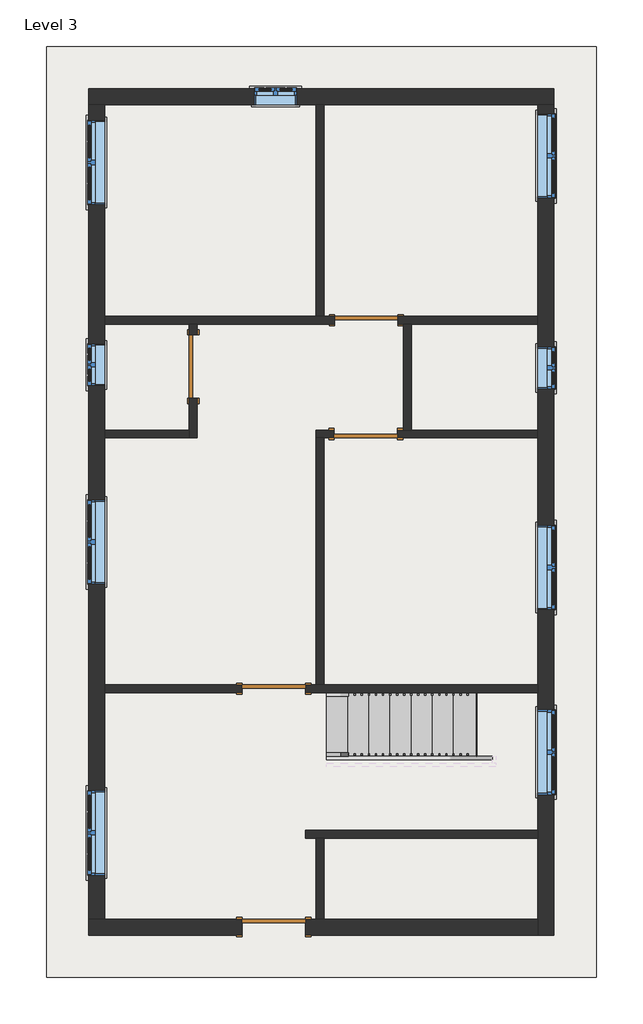
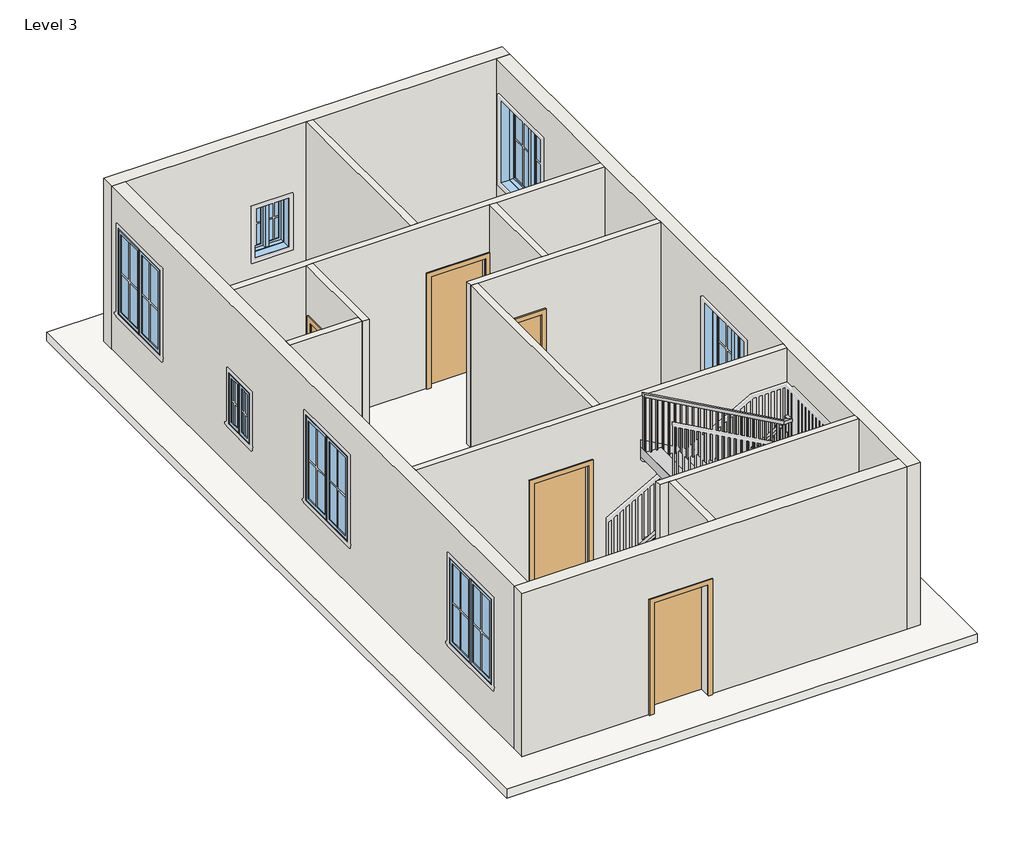
# One storey, part 1 of 2: 14 walls, 9 windows, 5 doors, 1 railing, 1 roof, 1 stair flight.
"""IFC4 building model written with IfcOpenShell, lengths in millimetres."""

from ifc_helpers import new_model, si_unit, frame, origin, place, context, project, spatial, polyline, outline, extrude, faceted_brep, transform, mapped, element, save
from components import door_305aa2a5, door_e5f9f3c4, door_a90ba1ad, stair_flight_ef7e9c63, window_c417fced, window_8377141f

model = new_model("IFC4")

# Units and contexts
model_context = context("Model", 3, world=origin())
ifc_project = project(units=[si_unit("LENGTHUNIT", "METRE", prefix="MILLI")], contexts=[model_context])

# Site, building, storey
site = spatial("IfcSite", under=ifc_project)
building = spatial("IfcBuilding", under=site)
storey = spatial("IfcBuildingStorey", under=building, Name="Level 3", Elevation=6096.0)

# Doors
placement = place(None, origin())
door_shape = door_305aa2a5(model_context)
element("IfcDoor", 1, ObjectType="Single-Flush : 36\" x 84\"", at=placement, inside=storey, context=model_context, shape_type="MappedRepresentation", body=[
    mapped(door_shape, transform((5270.5, 10636.25, 6096.0), x_axis=(-1.0, 0.0, 0.0), y_axis=(0.0, -1.0, 0.0), z_axis=(0.0, 0.0, 1.0))),
])
door_2_shape = door_e5f9f3c4(model_context)
element("IfcDoor", 2, ObjectType="Single-Flush : 36\" x 84\"", at=placement, inside=storey, context=model_context, shape_type="MappedRepresentation", body=[
    mapped(door_2_shape, transform((2774.95, 9969.5, 6096.0), x_axis=(0.0, 1.0, 0.0), y_axis=(-1.0, 0.0, 0.0), z_axis=(0.0, 0.0, 1.0))),
])
element("IfcDoor", 3, ObjectType="Single-Flush : 36\" x 84\"", at=placement, inside=storey, context=model_context, shape_type="MappedRepresentation", body=[
    mapped(door_2_shape, transform((5264.15, 8997.95, 6096.0), x_axis=(-1.0, 0.0, 0.0), y_axis=(0.0, -1.0, 0.0), z_axis=(0.0, 0.0, 1.0))),
])
element("IfcDoor", 4, ObjectType="Single-Flush : 36\" x 84\"", at=placement, inside=storey, context=model_context, shape_type="MappedRepresentation", body=[
    mapped(door_2_shape, transform((3937.0, 5327.65, 6096.0), x_axis=(1.0, 0.0, 0.0), y_axis=(0.0, 1.0, 0.0), z_axis=(0.0, 0.0, 1.0))),
])
door_3_shape = door_a90ba1ad(model_context)
element("IfcDoor", 5, ObjectType="Single-Flush : 36\" x 84\"", at=placement, inside=storey, context=model_context, shape_type="MappedRepresentation", body=[
    mapped(door_3_shape, transform((3937.0, 1892.3, 6096.0), x_axis=(-1.0, 0.0, 0.0), y_axis=(0.0, -1.0, 0.0), z_axis=(0.0, 0.0, 1.0))),
])

# Railing
element("IfcRailing", 6, ObjectType="Handrail - Rectangular", at=placement, inside=storey, context=model_context, shape_type="SolidModel", body=[
    faceted_brep([(4699.0, 4406.9, 7179.7333333), (4699.0, 4406.9, 7121.620221), (4699.0, 4356.1, 7121.620221), (4699.0, 4356.1, 7179.7333333), (7061.2, 4406.9, 8492.0666667), (7112.0, 4406.9, 8462.1757765), (7112.0, 4356.1, 8462.1757765), (7061.2, 4356.1, 8492.0666667), (7061.2, 4406.9, 8534.4), (7112.0, 4406.9, 8483.6), (7112.0, 4356.1, 8483.6), (7061.2, 4356.1, 8534.4), (7188.2, 4406.9, 8534.4), (7188.2, 4406.9, 8483.6), (7137.4, 4356.1, 8483.6), (7137.4, 4356.1, 8534.4), (7188.2, 4279.9, 8534.4), (7188.2, 4229.1, 8483.6), (7137.4, 4229.1, 8483.6), (7137.4, 4279.9, 8534.4), (7188.2, 4279.9, 8746.0666667), (7188.2, 4229.1, 8695.2666667), (7137.4, 4229.1, 8695.2666667), (7137.4, 4279.9, 8746.0666667), (7188.2, 4152.9, 8746.0666667), (7188.2, 4152.9, 8695.2666667), (7137.4, 4203.7, 8695.2666667), (7137.4, 4203.7, 8746.0666667), (7061.2, 4152.9, 8746.0666667), (7048.0363978, 4152.9, 8695.2666667), (7048.0363978, 4203.7, 8695.2666667), (7061.2, 4203.7, 8746.0666667), (4699.0, 4152.9, 10058.4), (4699.0, 4203.7, 10058.4), (4699.0, 4203.7, 10000.2868876), (4699.0, 4152.9, 10000.2868876)], [[[0, 1, 2, 3]], [[1, 0, 4, 5]], [[2, 1, 5, 6]], [[3, 2, 6, 7]], [[0, 3, 7, 4]], [[5, 4, 8, 9]], [[6, 5, 9, 10]], [[7, 6, 10, 11]], [[4, 7, 11, 8]], [[9, 8, 12, 13]], [[10, 9, 13, 14]], [[11, 10, 14, 15]], [[8, 11, 15, 12]], [[13, 12, 16, 17]], [[14, 13, 17, 18]], [[15, 14, 18, 19]], [[12, 15, 19, 16]], [[17, 16, 20, 21]], [[18, 17, 21, 22]], [[19, 18, 22, 23]], [[16, 19, 23, 20]], [[21, 20, 24, 25]], [[22, 21, 25, 26]], [[23, 22, 26, 27]], [[20, 23, 27, 24]], [[25, 24, 28, 29]], [[26, 25, 29, 30]], [[27, 26, 30, 31]], [[24, 27, 31, 28]], [[32, 33, 34, 35]], [[29, 28, 32, 35]], [[30, 29, 35, 34]], [[31, 30, 34, 33]], [[28, 31, 33, 32]]]),
    extrude(outline(polyline([(9980.8841099, 4733.925), (9991.4674432, 4714.875), (8974.6666667, 4714.875), (8974.6666667, 4733.925), (9980.8841099, 4733.925)])), frame((0.0, 4168.775, 0.0), z_axis=(0.0, 1.0, 0.0), x_axis=(0.0, 0.0, 1.0)), (0.0, 0.0, 1.0), 19.05),
    extrude(outline(polyline([(9924.4396654, 4835.525), (9935.0229988, 4816.475), (8974.6666667, 4816.475), (8974.6666667, 4835.525), (9924.4396654, 4835.525)])), frame((0.0, 4168.775, 0.0), z_axis=(0.0, 1.0, 0.0), x_axis=(0.0, 0.0, 1.0)), (0.0, 0.0, 1.0), 19.05),
    extrude(outline(polyline([(9867.995221, 4937.125), (9878.5785543, 4918.075), (8974.6666667, 4918.075), (8974.6666667, 4937.125), (9867.995221, 4937.125)])), frame((0.0, 4168.775, 0.0), z_axis=(0.0, 1.0, 0.0), x_axis=(0.0, 0.0, 1.0)), (0.0, 0.0, 1.0), 19.05),
    extrude(outline(polyline([(9811.5507765, 5038.725), (9822.1341099, 5019.675), (8805.3333333, 5019.675), (8805.3333333, 5038.725), (9811.5507765, 5038.725)])), frame((0.0, 4168.775, 0.0), z_axis=(0.0, 1.0, 0.0), x_axis=(0.0, 0.0, 1.0)), (0.0, 0.0, 1.0), 19.05),
    extrude(outline(polyline([(9755.1063321, 5140.325), (9765.6896654, 5121.275), (8805.3333333, 5121.275), (8805.3333333, 5140.325), (9755.1063321, 5140.325)])), frame((0.0, 4168.775, 0.0), z_axis=(0.0, 1.0, 0.0), x_axis=(0.0, 0.0, 1.0)), (0.0, 0.0, 1.0), 19.05),
    extrude(outline(polyline([(9698.6618876, 5241.925), (9709.245221, 5222.875), (8805.3333333, 5222.875), (8805.3333333, 5241.925), (9698.6618876, 5241.925)])), frame((0.0, 4168.775, 0.0), z_axis=(0.0, 1.0, 0.0), x_axis=(0.0, 0.0, 1.0)), (0.0, 0.0, 1.0), 19.05),
    extrude(outline(polyline([(9642.2174432, 5343.525), (9652.8007765, 5324.475), (8636.0, 5324.475), (8636.0, 5343.525), (9642.2174432, 5343.525)])), frame((0.0, 4168.775, 0.0), z_axis=(0.0, 1.0, 0.0), x_axis=(0.0, 0.0, 1.0)), (0.0, 0.0, 1.0), 19.05),
    extrude(outline(polyline([(9585.7729988, 5445.125), (9596.3563321, 5426.075), (8636.0, 5426.075), (8636.0, 5445.125), (9585.7729988, 5445.125)])), frame((0.0, 4168.775, 0.0), z_axis=(0.0, 1.0, 0.0), x_axis=(0.0, 0.0, 1.0)), (0.0, 0.0, 1.0), 19.05),
    extrude(outline(polyline([(9529.3285543, 5546.725), (9539.9118876, 5527.675), (8636.0, 5527.675), (8636.0, 5546.725), (9529.3285543, 5546.725)])), frame((0.0, 4168.775, 0.0), z_axis=(0.0, 1.0, 0.0), x_axis=(0.0, 0.0, 1.0)), (0.0, 0.0, 1.0), 19.05),
    extrude(outline(polyline([(9472.8841099, 5648.325), (9483.4674432, 5629.275), (8466.6666667, 5629.275), (8466.6666667, 5648.325), (9472.8841099, 5648.325)])), frame((0.0, 4168.775, 0.0), z_axis=(0.0, 1.0, 0.0), x_axis=(0.0, 0.0, 1.0)), (0.0, 0.0, 1.0), 19.05),
    extrude(outline(polyline([(9416.4396654, 5749.925), (9427.0229988, 5730.875), (8466.6666667, 5730.875), (8466.6666667, 5749.925), (9416.4396654, 5749.925)])), frame((0.0, 4168.775, 0.0), z_axis=(0.0, 1.0, 0.0), x_axis=(0.0, 0.0, 1.0)), (0.0, 0.0, 1.0), 19.05),
    extrude(outline(polyline([(9359.995221, 5851.525), (9370.5785543, 5832.475), (8466.6666667, 5832.475), (8466.6666667, 5851.525), (9359.995221, 5851.525)])), frame((0.0, 4168.775, 0.0), z_axis=(0.0, 1.0, 0.0), x_axis=(0.0, 0.0, 1.0)), (0.0, 0.0, 1.0), 19.05),
    extrude(outline(polyline([(9303.5507765, 5953.125), (9314.1341099, 5934.075), (8297.3333333, 5934.075), (8297.3333333, 5953.125), (9303.5507765, 5953.125)])), frame((0.0, 4168.775, 0.0), z_axis=(0.0, 1.0, 0.0), x_axis=(0.0, 0.0, 1.0)), (0.0, 0.0, 1.0), 19.05),
    extrude(outline(polyline([(9247.1063321, 6054.725), (9257.6896654, 6035.675), (8297.3333333, 6035.675), (8297.3333333, 6054.725), (9247.1063321, 6054.725)])), frame((0.0, 4168.775, 0.0), z_axis=(0.0, 1.0, 0.0), x_axis=(0.0, 0.0, 1.0)), (0.0, 0.0, 1.0), 19.05),
    extrude(outline(polyline([(9190.6618876, 6156.325), (9201.245221, 6137.275), (8297.3333333, 6137.275), (8297.3333333, 6156.325), (9190.6618876, 6156.325)])), frame((0.0, 4168.775, 0.0), z_axis=(0.0, 1.0, 0.0), x_axis=(0.0, 0.0, 1.0)), (0.0, 0.0, 1.0), 19.05),
    extrude(outline(polyline([(9134.2174432, 6257.925), (9144.8007765, 6238.875), (8128.0, 6238.875), (8128.0, 6257.925), (9134.2174432, 6257.925)])), frame((0.0, 4168.775, 0.0), z_axis=(0.0, 1.0, 0.0), x_axis=(0.0, 0.0, 1.0)), (0.0, 0.0, 1.0), 19.05),
    extrude(outline(polyline([(9077.7729988, 6359.525), (9088.3563321, 6340.475), (8128.0, 6340.475), (8128.0, 6359.525), (9077.7729988, 6359.525)])), frame((0.0, 4168.775, 0.0), z_axis=(0.0, 1.0, 0.0), x_axis=(0.0, 0.0, 1.0)), (0.0, 0.0, 1.0), 19.05),
    extrude(outline(polyline([(9021.3285543, 6461.125), (9031.9118876, 6442.075), (8128.0, 6442.075), (8128.0, 6461.125), (9021.3285543, 6461.125)])), frame((0.0, 4168.775, 0.0), z_axis=(0.0, 1.0, 0.0), x_axis=(0.0, 0.0, 1.0)), (0.0, 0.0, 1.0), 19.05),
    extrude(outline(polyline([(8964.8841099, 6562.725), (8975.4674432, 6543.675), (7958.6666667, 6543.675), (7958.6666667, 6562.725), (8964.8841099, 6562.725)])), frame((0.0, 4168.775, 0.0), z_axis=(0.0, 1.0, 0.0), x_axis=(0.0, 0.0, 1.0)), (0.0, 0.0, 1.0), 19.05),
    extrude(outline(polyline([(8908.4396654, 6664.325), (8919.0229988, 6645.275), (7958.6666667, 6645.275), (7958.6666667, 6664.325), (8908.4396654, 6664.325)])), frame((0.0, 4168.775, 0.0), z_axis=(0.0, 1.0, 0.0), x_axis=(0.0, 0.0, 1.0)), (0.0, 0.0, 1.0), 19.05),
    extrude(outline(polyline([(8851.995221, 6765.925), (8862.5785543, 6746.875), (7958.6666667, 6746.875), (7958.6666667, 6765.925), (8851.995221, 6765.925)])), frame((0.0, 4168.775, 0.0), z_axis=(0.0, 1.0, 0.0), x_axis=(0.0, 0.0, 1.0)), (0.0, 0.0, 1.0), 19.05),
    extrude(outline(polyline([(8795.5507765, 6867.525), (8806.1341099, 6848.475), (7789.3333333, 6848.475), (7789.3333333, 6867.525), (8795.5507765, 6867.525)])), frame((0.0, 4168.775, 0.0), z_axis=(0.0, 1.0, 0.0), x_axis=(0.0, 0.0, 1.0)), (0.0, 0.0, 1.0), 19.05),
    extrude(outline(polyline([(8739.1063321, 6969.125), (8749.6896654, 6950.075), (7789.3333333, 6950.075), (7789.3333333, 6969.125), (8739.1063321, 6969.125)])), frame((0.0, 4168.775, 0.0), z_axis=(0.0, 1.0, 0.0), x_axis=(0.0, 0.0, 1.0)), (0.0, 0.0, 1.0), 19.05),
    extrude(outline(polyline([(8682.6618876, 7070.725), (8693.245221, 7051.675), (7789.3333333, 7051.675), (7789.3333333, 7070.725), (8682.6618876, 7070.725)])), frame((0.0, 4168.775, 0.0), z_axis=(0.0, 1.0, 0.0), x_axis=(0.0, 0.0, 1.0)), (0.0, 0.0, 1.0), 19.05),
    extrude(outline(polyline([(7153.275, 4289.425), (7172.325, 4289.425), (7172.325, 4270.375), (7153.275, 4270.375), (7153.275, 4289.425)])), frame((0.0, 0.0, 7620.0), z_axis=(0.0, 0.0, 1.0), x_axis=(1.0, 0.0, 0.0)), (0.0, 0.0, 1.0), 863.6),
    extrude(outline(polyline([(7127.875, 4371.975), (7127.875, 4391.025), (7146.925, 4391.025), (7146.925, 4371.975), (7127.875, 4371.975)])), frame((0.0, 0.0, 7620.0), z_axis=(0.0, 0.0, 1.0), x_axis=(1.0, 0.0, 0.0)), (0.0, 0.0, 1.0), 863.6),
    extrude(outline(polyline([(8425.1341099, 7045.325), (8414.5507765, 7026.275), (7450.6666667, 7026.275), (7450.6666667, 7045.325), (8425.1341099, 7045.325)])), frame((0.0, 4371.975, 0.0), z_axis=(0.0, 1.0, 0.0), x_axis=(0.0, 0.0, 1.0)), (0.0, 0.0, 1.0), 19.05),
    extrude(outline(polyline([(8368.6896654, 6943.725), (8358.1063321, 6924.675), (7450.6666667, 6924.675), (7450.6666667, 6943.725), (8368.6896654, 6943.725)])), frame((0.0, 4371.975, 0.0), z_axis=(0.0, 1.0, 0.0), x_axis=(0.0, 0.0, 1.0)), (0.0, 0.0, 1.0), 19.05),
    extrude(outline(polyline([(8312.245221, 6842.125), (8301.6618876, 6823.075), (7450.6666667, 6823.075), (7450.6666667, 6842.125), (8312.245221, 6842.125)])), frame((0.0, 4371.975, 0.0), z_axis=(0.0, 1.0, 0.0), x_axis=(0.0, 0.0, 1.0)), (0.0, 0.0, 1.0), 19.05),
    extrude(outline(polyline([(8255.8007765, 6740.525), (8245.2174432, 6721.475), (7281.3333333, 6721.475), (7281.3333333, 6740.525), (8255.8007765, 6740.525)])), frame((0.0, 4371.975, 0.0), z_axis=(0.0, 1.0, 0.0), x_axis=(0.0, 0.0, 1.0)), (0.0, 0.0, 1.0), 19.05),
    extrude(outline(polyline([(8199.3563321, 6638.925), (8188.7729988, 6619.875), (7281.3333333, 6619.875), (7281.3333333, 6638.925), (8199.3563321, 6638.925)])), frame((0.0, 4371.975, 0.0), z_axis=(0.0, 1.0, 0.0), x_axis=(0.0, 0.0, 1.0)), (0.0, 0.0, 1.0), 19.05),
    extrude(outline(polyline([(8142.9118876, 6537.325), (8132.3285543, 6518.275), (7281.3333333, 6518.275), (7281.3333333, 6537.325), (8142.9118876, 6537.325)])), frame((0.0, 4371.975, 0.0), z_axis=(0.0, 1.0, 0.0), x_axis=(0.0, 0.0, 1.0)), (0.0, 0.0, 1.0), 19.05),
    extrude(outline(polyline([(8086.4674432, 6435.725), (8075.8841099, 6416.675), (7112.0, 6416.675), (7112.0, 6435.725), (8086.4674432, 6435.725)])), frame((0.0, 4371.975, 0.0), z_axis=(0.0, 1.0, 0.0), x_axis=(0.0, 0.0, 1.0)), (0.0, 0.0, 1.0), 19.05),
    extrude(outline(polyline([(8030.0229988, 6334.125), (8019.4396654, 6315.075), (7112.0, 6315.075), (7112.0, 6334.125), (8030.0229988, 6334.125)])), frame((0.0, 4371.975, 0.0), z_axis=(0.0, 1.0, 0.0), x_axis=(0.0, 0.0, 1.0)), (0.0, 0.0, 1.0), 19.05),
    extrude(outline(polyline([(7973.5785543, 6232.525), (7962.995221, 6213.475), (7112.0, 6213.475), (7112.0, 6232.525), (7973.5785543, 6232.525)])), frame((0.0, 4371.975, 0.0), z_axis=(0.0, 1.0, 0.0), x_axis=(0.0, 0.0, 1.0)), (0.0, 0.0, 1.0), 19.05),
    extrude(outline(polyline([(7917.1341099, 6130.925), (7906.5507765, 6111.875), (6942.6666667, 6111.875), (6942.6666667, 6130.925), (7917.1341099, 6130.925)])), frame((0.0, 4371.975, 0.0), z_axis=(0.0, 1.0, 0.0), x_axis=(0.0, 0.0, 1.0)), (0.0, 0.0, 1.0), 19.05),
    extrude(outline(polyline([(7860.6896654, 6029.325), (7850.1063321, 6010.275), (6942.6666667, 6010.275), (6942.6666667, 6029.325), (7860.6896654, 6029.325)])), frame((0.0, 4371.975, 0.0), z_axis=(0.0, 1.0, 0.0), x_axis=(0.0, 0.0, 1.0)), (0.0, 0.0, 1.0), 19.05),
    extrude(outline(polyline([(7804.245221, 5927.725), (7793.6618876, 5908.675), (6942.6666667, 5908.675), (6942.6666667, 5927.725), (7804.245221, 5927.725)])), frame((0.0, 4371.975, 0.0), z_axis=(0.0, 1.0, 0.0), x_axis=(0.0, 0.0, 1.0)), (0.0, 0.0, 1.0), 19.05),
    extrude(outline(polyline([(7747.8007765, 5826.125), (7737.2174432, 5807.075), (6773.3333333, 5807.075), (6773.3333333, 5826.125), (7747.8007765, 5826.125)])), frame((0.0, 4371.975, 0.0), z_axis=(0.0, 1.0, 0.0), x_axis=(0.0, 0.0, 1.0)), (0.0, 0.0, 1.0), 19.05),
    extrude(outline(polyline([(7691.3563321, 5724.525), (7680.7729988, 5705.475), (6773.3333333, 5705.475), (6773.3333333, 5724.525), (7691.3563321, 5724.525)])), frame((0.0, 4371.975, 0.0), z_axis=(0.0, 1.0, 0.0), x_axis=(0.0, 0.0, 1.0)), (0.0, 0.0, 1.0), 19.05),
    extrude(outline(polyline([(7634.9118876, 5622.925), (7624.3285543, 5603.875), (6773.3333333, 5603.875), (6773.3333333, 5622.925), (7634.9118876, 5622.925)])), frame((0.0, 4371.975, 0.0), z_axis=(0.0, 1.0, 0.0), x_axis=(0.0, 0.0, 1.0)), (0.0, 0.0, 1.0), 19.05),
    extrude(outline(polyline([(7578.4674432, 5521.325), (7567.8841099, 5502.275), (6604.0, 5502.275), (6604.0, 5521.325), (7578.4674432, 5521.325)])), frame((0.0, 4371.975, 0.0), z_axis=(0.0, 1.0, 0.0), x_axis=(0.0, 0.0, 1.0)), (0.0, 0.0, 1.0), 19.05),
    extrude(outline(polyline([(7522.0229988, 5419.725), (7511.4396654, 5400.675), (6604.0, 5400.675), (6604.0, 5419.725), (7522.0229988, 5419.725)])), frame((0.0, 4371.975, 0.0), z_axis=(0.0, 1.0, 0.0), x_axis=(0.0, 0.0, 1.0)), (0.0, 0.0, 1.0), 19.05),
    extrude(outline(polyline([(7465.5785543, 5318.125), (7454.995221, 5299.075), (6604.0, 5299.075), (6604.0, 5318.125), (7465.5785543, 5318.125)])), frame((0.0, 4371.975, 0.0), z_axis=(0.0, 1.0, 0.0), x_axis=(0.0, 0.0, 1.0)), (0.0, 0.0, 1.0), 19.05),
    extrude(outline(polyline([(7409.1341099, 5216.525), (7398.5507765, 5197.475), (6434.6666667, 5197.475), (6434.6666667, 5216.525), (7409.1341099, 5216.525)])), frame((0.0, 4371.975, 0.0), z_axis=(0.0, 1.0, 0.0), x_axis=(0.0, 0.0, 1.0)), (0.0, 0.0, 1.0), 19.05),
    extrude(outline(polyline([(7352.6896654, 5114.925), (7342.1063321, 5095.875), (6434.6666667, 5095.875), (6434.6666667, 5114.925), (7352.6896654, 5114.925)])), frame((0.0, 4371.975, 0.0), z_axis=(0.0, 1.0, 0.0), x_axis=(0.0, 0.0, 1.0)), (0.0, 0.0, 1.0), 19.05),
    extrude(outline(polyline([(7296.245221, 5013.325), (7285.6618876, 4994.275), (6434.6666667, 4994.275), (6434.6666667, 5013.325), (7296.245221, 5013.325)])), frame((0.0, 4371.975, 0.0), z_axis=(0.0, 1.0, 0.0), x_axis=(0.0, 0.0, 1.0)), (0.0, 0.0, 1.0), 19.05),
    extrude(outline(polyline([(7239.8007765, 4911.725), (7229.2174432, 4892.675), (6265.3333333, 4892.675), (6265.3333333, 4911.725), (7239.8007765, 4911.725)])), frame((0.0, 4371.975, 0.0), z_axis=(0.0, 1.0, 0.0), x_axis=(0.0, 0.0, 1.0)), (0.0, 0.0, 1.0), 19.05),
    extrude(outline(polyline([(7183.3563321, 4810.125), (7172.7729988, 4791.075), (6265.3333333, 4791.075), (6265.3333333, 4810.125), (7183.3563321, 4810.125)])), frame((0.0, 4371.975, 0.0), z_axis=(0.0, 1.0, 0.0), x_axis=(0.0, 0.0, 1.0)), (0.0, 0.0, 1.0), 19.05),
    extrude(outline(polyline([(7153.275, 4187.825), (7172.325, 4187.825), (7172.325, 4168.775), (7153.275, 4168.775), (7153.275, 4187.825)])), frame((0.0, 0.0, 7620.0), z_axis=(0.0, 0.0, 1.0), x_axis=(1.0, 0.0, 0.0)), (0.0, 0.0, 1.0), 1075.2666667),
    extrude(outline(polyline([(7153.275, 4371.975), (7153.275, 4391.025), (7172.325, 4391.025), (7172.325, 4371.975), (7153.275, 4371.975)])), frame((0.0, 0.0, 7620.0), z_axis=(0.0, 0.0, 1.0), x_axis=(1.0, 0.0, 0.0)), (0.0, 0.0, 1.0), 863.6),
    extrude(outline(polyline([(9989.7035543, 4718.05), (10000.2868876, 4699.0), (8974.6666667, 4699.0), (8974.6666667, 4718.05), (9989.7035543, 4718.05)])), frame((0.0, 4168.775, 0.0), z_axis=(0.0, 1.0, 0.0), x_axis=(0.0, 0.0, 1.0)), (0.0, 0.0, 1.0), 19.05),
    extrude(outline(polyline([(7132.2035543, 4718.05), (7121.620221, 4699.0), (6265.3333333, 4699.0), (6265.3333333, 4718.05), (7132.2035543, 4718.05)])), frame((0.0, 4371.975, 0.0), z_axis=(0.0, 1.0, 0.0), x_axis=(0.0, 0.0, 1.0)), (0.0, 0.0, 1.0), 19.05),
])

# Roof
element("IfcRoof", 7, ObjectType="Generic - 12\"", at=placement, inside=storey, context=model_context, shape_type="SweptSolid", body=[
    extrude(outline(polyline([(660.4, 14579.6), (8585.2, 14579.6), (8585.2, 1168.4), (660.4, 1168.4), (660.4, 14579.6)])), frame((0.0, 0.0, 6096.0), z_axis=(0.0, 0.0, 1.0), x_axis=(1.0, 0.0, 0.0)), (0.0, 0.0, 1.0), 152.4),
])

# Stair flight
stair_flight_shape = stair_flight_ef7e9c63(model_context)
element("IfcStairFlight", 8, ObjectType="2\" Tread 1\" Nosing 1/4\" Riser", at=placement, inside=storey, context=model_context, shape_type="MappedRepresentation", body=[
    mapped(stair_flight_shape, transform((0.0, 0.0, 0.0), x_axis=(1.0, 0.0, 0.0), y_axis=(0.0, 1.0, 0.0), z_axis=(0.0, 0.0, 1.0))),
])

# Walls
element("IfcWall", 9, ObjectType="Generic - 5\"", at=placement, inside=storey, context=model_context, shape_type="SweptSolid", body=[
    extrude(outline(polyline([(4546.6, 10693.4), (4546.6, 13741.4), (4660.9, 13741.4), (4660.9, 10693.4), (4546.6, 10693.4)])), frame((0.0, 0.0, 6096.0), z_axis=(0.0, 0.0, 1.0), x_axis=(1.0, 0.0, 0.0)), (0.0, 0.0, 1.0), 3048.0),
])
element("IfcWall", 10, ObjectType="Generic - 5\"", at=placement, inside=storey, context=model_context, shape_type="Brep", body=[
    faceted_brep([(1498.6, 10579.1, 6096.0), (2717.8, 10579.1, 6096.0), (2832.1, 10579.1, 6096.0), (4813.3, 10579.1, 6096.0), (4813.3, 10579.1, 8229.6), (5727.7, 10579.1, 8229.6), (5727.7, 10579.1, 6096.0), (5803.9, 10579.1, 6096.0), (5918.2, 10579.1, 6096.0), (7747.0, 10579.1, 6096.0), (7747.0, 10579.1, 9144.0), (5918.2, 10579.1, 9144.0), (5803.9, 10579.1, 9144.0), (2832.1, 10579.1, 9144.0), (2717.8, 10579.1, 9144.0), (1498.6, 10579.1, 9144.0), (4813.3, 10693.4, 8229.6), (4813.3, 10693.4, 6096.0), (4660.9, 10693.4, 6096.0), (4546.6, 10693.4, 6096.0), (1498.6, 10693.4, 6096.0), (1498.6, 10693.4, 9144.0), (4546.6, 10693.4, 9144.0), (4660.9, 10693.4, 9144.0), (7747.0, 10693.4, 9144.0), (7747.0, 10693.4, 6096.0), (5727.7, 10693.4, 6096.0), (5727.7, 10693.4, 8229.6)], [[[0, 1, 2, 3, 4, 5, 6, 7, 8, 9, 10, 11, 12, 13, 14, 15]], [[16, 17, 18, 19, 20, 21, 22, 23, 24, 25, 26, 27]], [[26, 25, 9, 8, 7, 6]], [[20, 19, 18, 17, 3, 2, 1, 0]], [[15, 14, 13, 12, 11, 10, 24, 23, 22, 21]], [[10, 9, 25, 24]], [[0, 15, 21, 20]], [[4, 3, 17, 16]], [[5, 4, 16, 27]], [[6, 5, 27, 26]]]),
])
element("IfcWall", 11, ObjectType="Generic - 5\"", at=placement, inside=storey, context=model_context, shape_type="Brep", body=[
    faceted_brep([(2717.8, 10579.1, 6096.0), (2717.8, 10426.7, 6096.0), (2717.8, 10426.7, 8229.6), (2717.8, 9512.3, 8229.6), (2717.8, 9512.3, 6096.0), (2717.8, 9055.1, 6096.0), (2717.8, 8940.8, 6096.0), (2717.8, 8940.8, 9144.0), (2717.8, 9055.1, 9144.0), (2717.8, 10579.1, 9144.0), (2832.1, 10426.7, 8229.6), (2832.1, 10426.7, 6096.0), (2832.1, 10579.1, 6096.0), (2832.1, 10579.1, 9144.0), (2832.1, 8940.8, 9144.0), (2832.1, 8940.8, 6096.0), (2832.1, 9512.3, 6096.0), (2832.1, 9512.3, 8229.6)], [[[0, 1, 2, 3, 4, 5, 6, 7, 8, 9]], [[10, 11, 12, 13, 14, 15, 16, 17]], [[16, 15, 6, 5, 4]], [[12, 11, 1, 0]], [[9, 8, 7, 14, 13]], [[0, 9, 13, 12]], [[7, 6, 15, 14]], [[2, 1, 11, 10]], [[3, 2, 10, 17]], [[4, 3, 17, 16]]]),
])
element("IfcWall", 12, ObjectType="Generic - 5\"", at=placement, inside=storey, context=model_context, shape_type="SweptSolid", body=[
    extrude(outline(polyline([(2717.8, 8940.8), (1498.6, 8940.8), (1498.6, 9055.1), (2717.8, 9055.1), (2717.8, 8940.8)])), frame((0.0, 0.0, 6096.0), z_axis=(0.0, 0.0, 1.0), x_axis=(1.0, 0.0, 0.0)), (0.0, 0.0, 1.0), 3048.0),
])
element("IfcWall", 13, ObjectType="Generic - 5\"", at=placement, inside=storey, context=model_context, shape_type="SweptSolid", body=[
    extrude(outline(polyline([(5803.9, 9055.1), (5803.9, 10579.1), (5918.2, 10579.1), (5918.2, 9055.1), (5803.9, 9055.1)])), frame((0.0, 0.0, 6096.0), z_axis=(0.0, 0.0, 1.0), x_axis=(1.0, 0.0, 0.0)), (0.0, 0.0, 1.0), 3048.0),
])
element("IfcWall", 14, ObjectType="Generic - 5\"", at=placement, inside=storey, context=model_context, shape_type="Brep", body=[
    faceted_brep([(4806.95, 9055.1, 8229.6), (4806.95, 9055.1, 6096.0), (4546.6, 9055.1, 6096.0), (4546.6, 9055.1, 9144.0), (5803.9, 9055.1, 9144.0), (5918.2, 9055.1, 9144.0), (7747.0, 9055.1, 9144.0), (7747.0, 9055.1, 6096.0), (5918.2, 9055.1, 6096.0), (5803.9, 9055.1, 6096.0), (5721.35, 9055.1, 6096.0), (5721.35, 9055.1, 8229.6), (4546.6, 8940.8, 6096.0), (4660.9, 8940.8, 6096.0), (4806.95, 8940.8, 6096.0), (4806.95, 8940.8, 8229.6), (5721.35, 8940.8, 8229.6), (5721.35, 8940.8, 6096.0), (7747.0, 8940.8, 6096.0), (7747.0, 8940.8, 9144.0), (4660.9, 8940.8, 9144.0), (4546.6, 8940.8, 9144.0)], [[[0, 1, 2, 3, 4, 5, 6, 7, 8, 9, 10, 11]], [[12, 13, 14, 15, 16, 17, 18, 19, 20, 21]], [[2, 1, 14, 13, 12]], [[10, 9, 8, 7, 18, 17]], [[6, 5, 4, 3, 21, 20, 19]], [[7, 6, 19, 18]], [[3, 2, 12, 21]], [[15, 14, 1, 0]], [[16, 15, 0, 11]], [[17, 16, 11, 10]]]),
])
element("IfcWall", 15, ObjectType="Generic - 5\"", at=placement, inside=storey, context=model_context, shape_type="Brep", body=[
    faceted_brep([(4394.2, 5270.5, 8229.6), (4394.2, 5270.5, 6096.0), (7747.0, 5270.5, 6096.0), (7747.0, 5270.5, 9144.0), (1498.6, 5270.5, 9144.0), (1498.6, 5270.5, 6096.0), (3479.8, 5270.5, 6096.0), (3479.8, 5270.5, 8229.6), (7747.0, 5384.8, 6096.0), (4660.9, 5384.8, 6096.0), (4546.6, 5384.8, 6096.0), (4394.2, 5384.8, 6096.0), (4394.2, 5384.8, 8229.6), (3479.8, 5384.8, 8229.6), (3479.8, 5384.8, 6096.0), (1498.6, 5384.8, 6096.0), (1498.6, 5384.8, 9144.0), (4546.6, 5384.8, 9144.0), (4660.9, 5384.8, 9144.0), (7747.0, 5384.8, 9144.0)], [[[0, 1, 2, 3, 4, 5, 6, 7]], [[8, 9, 10, 11, 12, 13, 14, 15, 16, 17, 18, 19]], [[6, 5, 15, 14]], [[2, 1, 11, 10, 9, 8]], [[4, 3, 19, 18, 17, 16]], [[3, 2, 8, 19]], [[5, 4, 16, 15]], [[12, 11, 1, 0]], [[13, 12, 0, 7]], [[14, 13, 7, 6]]]),
])
element("IfcWall", 16, ObjectType="Generic - 5\"", at=placement, inside=storey, context=model_context, shape_type="SweptSolid", body=[
    extrude(outline(polyline([(4660.9, 8940.8), (4660.9, 5384.8), (4546.6, 5384.8), (4546.6, 8940.8), (4660.9, 8940.8)])), frame((0.0, 0.0, 6096.0), z_axis=(0.0, 0.0, 1.0), x_axis=(1.0, 0.0, 0.0)), (0.0, 0.0, 1.0), 3048.0),
])
element("IfcWall", 17, ObjectType="Generic - 5\"", at=placement, inside=storey, context=model_context, shape_type="SweptSolid", body=[
    extrude(outline(polyline([(4660.9, 3175.0), (4660.9, 2006.6), (4546.6, 2006.6), (4546.6, 3175.0), (4660.9, 3175.0)])), frame((0.0, 0.0, 6096.0), z_axis=(0.0, 0.0, 1.0), x_axis=(1.0, 0.0, 0.0)), (0.0, 0.0, 1.0), 3048.0),
])
element("IfcWall", 18, ObjectType="Generic - 5\"", at=placement, inside=storey, context=model_context, shape_type="Brep", body=[
    faceted_brep([(4394.2, 3175.0, 6096.0), (4546.6, 3175.0, 6096.0), (4660.9, 3175.0, 6096.0), (7747.0, 3175.0, 6096.0), (7747.0, 3175.0, 9144.0), (4660.9, 3175.0, 9144.0), (4546.6, 3175.0, 9144.0), (4394.2, 3175.0, 9144.0), (4394.2, 3289.3, 6096.0), (4394.2, 3289.3, 9144.0), (7747.0, 3289.3, 9144.0), (7747.0, 3289.3, 6096.0)], [[[0, 1, 2, 3, 4, 5, 6, 7]], [[8, 9, 10, 11]], [[3, 2, 1, 0, 8, 11]], [[7, 6, 5, 4, 10, 9]], [[0, 7, 9, 8]], [[4, 3, 11, 10]]]),
])
element("IfcWall", 19, ObjectType="Generic - 8\"", at=placement, inside=storey, context=model_context, shape_type="Brep", body=[
    faceted_brep([(1270.0, 13741.4, 6096.0), (1498.6, 13741.4, 6096.0), (4546.6, 13741.4, 6096.0), (4660.9, 13741.4, 6096.0), (7747.0, 13741.4, 6096.0), (7975.6, 13741.4, 6096.0), (7975.6, 13741.4, 9144.0), (7747.0, 13741.4, 9144.0), (4660.9, 13741.4, 9144.0), (4546.6, 13741.4, 9144.0), (1498.6, 13741.4, 9144.0), (1270.0, 13741.4, 9144.0), (4267.2, 13741.4, 7924.8), (4267.2, 13741.4, 7010.4), (3657.6, 13741.4, 7010.4), (3657.6, 13741.4, 7924.8), (1270.0, 13970.0, 6096.0), (1270.0, 13970.0, 9144.0), (7975.6, 13970.0, 9144.0), (7975.6, 13970.0, 6096.0), (4267.2, 13970.0, 7924.8), (3657.6, 13970.0, 7924.8), (3657.6, 13970.0, 7010.4), (4267.2, 13970.0, 7010.4)], [[[0, 1, 2, 3, 4, 5, 6, 7, 8, 9, 10, 11], [12, 13, 14, 15]], [[16, 17, 18, 19], [20, 21, 22, 23]], [[5, 4, 3, 2, 1, 0, 16, 19]], [[11, 10, 9, 8, 7, 6, 18, 17]], [[6, 5, 19, 18]], [[0, 11, 17, 16]], [[13, 12, 20, 23]], [[14, 13, 23, 22]], [[15, 14, 22, 21]], [[12, 15, 21, 20]]]),
])
element("IfcWall", 20, ObjectType="Generic - 8\"", at=placement, inside=storey, context=model_context, shape_type="Brep", body=[
    faceted_brep([(7747.0, 13741.4, 6096.0), (7747.0, 10693.4, 6096.0), (7747.0, 10579.1, 6096.0), (7747.0, 9055.1, 6096.0), (7747.0, 8940.8, 6096.0), (7747.0, 5384.8, 6096.0), (7747.0, 5270.5, 6096.0), (7747.0, 3289.3, 6096.0), (7747.0, 3175.0, 6096.0), (7747.0, 2006.6, 6096.0), (7747.0, 1778.0, 6096.0), (7747.0, 1778.0, 9144.0), (7747.0, 2006.6, 9144.0), (7747.0, 3175.0, 9144.0), (7747.0, 3289.3, 9144.0), (7747.0, 5270.5, 9144.0), (7747.0, 5384.8, 9144.0), (7747.0, 8940.8, 9144.0), (7747.0, 9055.1, 9144.0), (7747.0, 10579.1, 9144.0), (7747.0, 10693.4, 9144.0), (7747.0, 13741.4, 9144.0), (7747.0, 12395.2, 8534.4), (7747.0, 12395.2, 7010.4), (7747.0, 13614.4, 7010.4), (7747.0, 13614.4, 8534.4), (7747.0, 6464.3, 8534.4), (7747.0, 6464.3, 7010.4), (7747.0, 7683.5, 7010.4), (7747.0, 7683.5, 8534.4), (7747.0, 9645.65, 7924.8), (7747.0, 9645.65, 7010.4), (7747.0, 10255.25, 7010.4), (7747.0, 10255.25, 7924.8), (7747.0, 3803.65, 8534.4), (7747.0, 3803.65, 7010.4), (7747.0, 5022.85, 7010.4), (7747.0, 5022.85, 8534.4), (7975.6, 13741.4, 6096.0), (7975.6, 13741.4, 9144.0), (7975.6, 1778.0, 9144.0), (7975.6, 1778.0, 6096.0), (7975.6, 12395.2, 8534.4), (7975.6, 13614.4, 8534.4), (7975.6, 13614.4, 7010.4), (7975.6, 12395.2, 7010.4), (7975.6, 6464.3, 8534.4), (7975.6, 7683.5, 8534.4), (7975.6, 7683.5, 7010.4), (7975.6, 6464.3, 7010.4), (7975.6, 9645.65, 7924.8), (7975.6, 10255.25, 7924.8), (7975.6, 10255.25, 7010.4), (7975.6, 9645.65, 7010.4), (7975.6, 3803.65, 8534.4), (7975.6, 5022.85, 8534.4), (7975.6, 5022.85, 7010.4), (7975.6, 3803.65, 7010.4)], [[[0, 1, 2, 3, 4, 5, 6, 7, 8, 9, 10, 11, 12, 13, 14, 15, 16, 17, 18, 19, 20, 21], [22, 23, 24, 25], [26, 27, 28, 29], [30, 31, 32, 33], [34, 35, 36, 37]], [[38, 39, 40, 41], [42, 43, 44, 45], [46, 47, 48, 49], [50, 51, 52, 53], [54, 55, 56, 57]], [[10, 9, 8, 7, 6, 5, 4, 3, 2, 1, 0, 38, 41]], [[21, 20, 19, 18, 17, 16, 15, 14, 13, 12, 11, 40, 39]], [[0, 21, 39, 38]], [[11, 10, 41, 40]], [[23, 22, 42, 45]], [[24, 23, 45, 44]], [[25, 24, 44, 43]], [[22, 25, 43, 42]], [[27, 26, 46, 49]], [[28, 27, 49, 48]], [[29, 28, 48, 47]], [[26, 29, 47, 46]], [[31, 30, 50, 53]], [[32, 31, 53, 52]], [[33, 32, 52, 51]], [[30, 33, 51, 50]], [[35, 34, 54, 57]], [[36, 35, 57, 56]], [[37, 36, 56, 55]], [[34, 37, 55, 54]]]),
])
element("IfcWall", 21, ObjectType="Generic - 8\"", at=placement, inside=storey, context=model_context, shape_type="Brep", body=[
    faceted_brep([(3479.8, 2006.6, 8229.6), (3479.8, 2006.6, 6096.0), (1498.6, 2006.6, 6096.0), (1270.0, 2006.6, 6096.0), (1270.0, 2006.6, 9144.0), (1498.6, 2006.6, 9144.0), (4546.6, 2006.6, 9144.0), (4660.9, 2006.6, 9144.0), (7747.0, 2006.6, 9144.0), (7747.0, 2006.6, 6096.0), (4660.9, 2006.6, 6096.0), (4546.6, 2006.6, 6096.0), (4394.2, 2006.6, 6096.0), (4394.2, 2006.6, 8229.6), (1270.0, 1778.0, 6096.0), (3479.8, 1778.0, 6096.0), (3479.8, 1778.0, 8229.6), (4394.2, 1778.0, 8229.6), (4394.2, 1778.0, 6096.0), (7747.0, 1778.0, 6096.0), (7747.0, 1778.0, 9144.0), (1270.0, 1778.0, 9144.0)], [[[0, 1, 2, 3, 4, 5, 6, 7, 8, 9, 10, 11, 12, 13]], [[14, 15, 16, 17, 18, 19, 20, 21]], [[3, 2, 1, 15, 14]], [[12, 11, 10, 9, 19, 18]], [[8, 7, 6, 5, 4, 21, 20]], [[9, 8, 20, 19]], [[4, 3, 14, 21]], [[16, 15, 1, 0]], [[17, 16, 0, 13]], [[18, 17, 13, 12]]]),
])
element("IfcWall", 22, ObjectType="Generic - 8\"", at=placement, inside=storey, context=model_context, shape_type="Brep", body=[
    faceted_brep([(1498.6, 2006.6, 6096.0), (1498.6, 5270.5, 6096.0), (1498.6, 5384.8, 6096.0), (1498.6, 8940.8, 6096.0), (1498.6, 9055.1, 6096.0), (1498.6, 10579.1, 6096.0), (1498.6, 10693.4, 6096.0), (1498.6, 13741.4, 6096.0), (1498.6, 13741.4, 9144.0), (1498.6, 10693.4, 9144.0), (1498.6, 10579.1, 9144.0), (1498.6, 9055.1, 9144.0), (1498.6, 8940.8, 9144.0), (1498.6, 5384.8, 9144.0), (1498.6, 5270.5, 9144.0), (1498.6, 2006.6, 9144.0), (1498.6, 3860.3039063, 8534.4), (1498.6, 3860.3039063, 7010.4), (1498.6, 2641.1039063, 7010.4), (1498.6, 2641.1039063, 8534.4), (1498.6, 8051.3039062, 8534.4), (1498.6, 8051.3039062, 7010.4), (1498.6, 6832.1039062, 7010.4), (1498.6, 6832.1039062, 8534.4), (1498.6, 13518.6539062, 8534.4), (1498.6, 13518.6539062, 7010.4), (1498.6, 12299.4539062, 7010.4), (1498.6, 12299.4539062, 8534.4), (1498.6, 10299.2039062, 7924.8), (1498.6, 10299.2039062, 7010.4), (1498.6, 9689.6039062, 7010.4), (1498.6, 9689.6039062, 7924.8), (1270.0, 2006.6, 6096.0), (1270.0, 2006.6, 9144.0), (1270.0, 13741.4, 9144.0), (1270.0, 13741.4, 6096.0), (1270.0, 3860.3039063, 8534.4), (1270.0, 2641.1039063, 8534.4), (1270.0, 2641.1039063, 7010.4), (1270.0, 3860.3039063, 7010.4), (1270.0, 8051.3039062, 8534.4), (1270.0, 6832.1039062, 8534.4), (1270.0, 6832.1039062, 7010.4), (1270.0, 8051.3039062, 7010.4), (1270.0, 13518.6539062, 8534.4), (1270.0, 12299.4539062, 8534.4), (1270.0, 12299.4539062, 7010.4), (1270.0, 13518.6539062, 7010.4), (1270.0, 10299.2039062, 7924.8), (1270.0, 9689.6039062, 7924.8), (1270.0, 9689.6039062, 7010.4), (1270.0, 10299.2039062, 7010.4)], [[[0, 1, 2, 3, 4, 5, 6, 7, 8, 9, 10, 11, 12, 13, 14, 15], [16, 17, 18, 19], [20, 21, 22, 23], [24, 25, 26, 27], [28, 29, 30, 31]], [[32, 33, 34, 35], [36, 37, 38, 39], [40, 41, 42, 43], [44, 45, 46, 47], [48, 49, 50, 51]], [[7, 6, 5, 4, 3, 2, 1, 0, 32, 35]], [[15, 14, 13, 12, 11, 10, 9, 8, 34, 33]], [[0, 15, 33, 32]], [[8, 7, 35, 34]], [[17, 16, 36, 39]], [[18, 17, 39, 38]], [[19, 18, 38, 37]], [[16, 19, 37, 36]], [[21, 20, 40, 43]], [[22, 21, 43, 42]], [[23, 22, 42, 41]], [[20, 23, 41, 40]], [[25, 24, 44, 47]], [[26, 25, 47, 46]], [[27, 26, 46, 45]], [[24, 27, 45, 44]], [[29, 28, 48, 51]], [[30, 29, 51, 50]], [[31, 30, 50, 49]], [[28, 31, 49, 48]]]),
])

# Windows
window_shape = window_c417fced(model_context)
element("IfcWindow", 23, ObjectType="Window-Casement-Double : 24\" x 36\"", at=placement, inside=storey, context=model_context, shape_type="MappedRepresentation", body=[
    mapped(window_shape, transform((3962.4, 13855.7, 6096.0), x_axis=(1.0, 0.0, 0.0), y_axis=(0.0, 1.0, 0.0), z_axis=(0.0, 0.0, 1.0))),
])
element("IfcWindow", 24, ObjectType="Window-Casement-Double : 24\" x 36\"", at=placement, inside=storey, context=model_context, shape_type="MappedRepresentation", body=[
    mapped(window_shape, transform((7861.3, 9950.45, 6096.0), x_axis=(0.0, -1.0, 0.0), y_axis=(1.0, 0.0, 0.0), z_axis=(0.0, 0.0, 1.0))),
])
element("IfcWindow", 25, ObjectType="Window-Casement-Double : 24\" x 36\"", at=placement, inside=storey, context=model_context, shape_type="MappedRepresentation", body=[
    mapped(window_shape, transform((1384.3, 9994.4039062, 6096.0), x_axis=(0.0, 1.0, 0.0), y_axis=(-1.0, 0.0, 0.0), z_axis=(0.0, 0.0, 1.0))),
])
window_2_shape = window_8377141f(model_context)
element("IfcWindow", 26, ObjectType="Window-Casement-Double : 48\" x 60\"", at=placement, inside=storey, context=model_context, shape_type="MappedRepresentation", body=[
    mapped(window_2_shape, transform((1384.3, 3250.7039063, 6096.0), x_axis=(0.0, 1.0, 0.0), y_axis=(-1.0, 0.0, 0.0), z_axis=(0.0, 0.0, 1.0))),
])
element("IfcWindow", 27, ObjectType="Window-Casement-Double : 48\" x 60\"", at=placement, inside=storey, context=model_context, shape_type="MappedRepresentation", body=[
    mapped(window_2_shape, transform((1384.3, 7441.7039063, 6096.0), x_axis=(0.0, 1.0, 0.0), y_axis=(-1.0, 0.0, 0.0), z_axis=(0.0, 0.0, 1.0))),
])
element("IfcWindow", 28, ObjectType="Window-Casement-Double : 48\" x 60\"", at=placement, inside=storey, context=model_context, shape_type="MappedRepresentation", body=[
    mapped(window_2_shape, transform((1384.3, 12909.0539063, 6096.0), x_axis=(0.0, 1.0, 0.0), y_axis=(-1.0, 0.0, 0.0), z_axis=(0.0, 0.0, 1.0))),
])
element("IfcWindow", 29, ObjectType="Window-Casement-Double : 48\" x 60\"", at=placement, inside=storey, context=model_context, shape_type="MappedRepresentation", body=[
    mapped(window_2_shape, transform((7861.3, 13004.8, 6096.0), x_axis=(0.0, -1.0, 0.0), y_axis=(1.0, 0.0, 0.0), z_axis=(0.0, 0.0, 1.0))),
])
element("IfcWindow", 30, ObjectType="Window-Casement-Double : 48\" x 60\"", at=placement, inside=storey, context=model_context, shape_type="MappedRepresentation", body=[
    mapped(window_2_shape, transform((7861.3, 7073.9, 6096.0), x_axis=(0.0, -1.0, 0.0), y_axis=(1.0, 0.0, 0.0), z_axis=(0.0, 0.0, 1.0))),
])
element("IfcWindow", 31, ObjectType="Window-Casement-Double : 48\" x 60\"", at=placement, inside=storey, context=model_context, shape_type="MappedRepresentation", body=[
    mapped(window_2_shape, transform((7861.3, 4413.25, 6096.0), x_axis=(0.0, -1.0, 0.0), y_axis=(1.0, 0.0, 0.0), z_axis=(0.0, 0.0, 1.0))),
])

save(model, "model.ifc")

# Revit data of these elements
# Type "Single-Flush : 36\" x 84\""
#   Type Mark = "1"
#   Construction Type Id = "MDOOR"
#   Assembly Code = "C1020"
#   Analytic Construction = "Metal"
#   Thickness = 0' - 2"
#   Heat Transfer Coefficient (U) = 0.651978 BTU/(h·ft²·°F)
#   Height = 7' - 0"
#   Trim Projection Ext = 0' - 1"
#   Trim Projection Int = 0' - 1"
#   Trim Width = 0' - 3"
#   Width = 3' - 0"
#   Define Thermal Properties by = 1
#   Define Thermal Properties by = 1
#   Door Material = Door - Panel
#   Frame Material = Door - Frame
#   Visual Light Transmittance = 0
#   Solar Heat Gain Coefficient = 0
#   Function = (empty or 0)
#   Wall Closure = (empty or 0)
# Type "Handrail - Rectangular"
#   Assembly Code = "C2010400"
#   built-in parameter 1008612 = 0.0416667 (stored number, unit not read)
#   built-in parameter 1008611 = 0.0416667 (stored number, unit not read)
#   built-in parameter 1008609 = 0.333333 (stored number, unit not read)
#   built-in parameter 1008604 = 0.166667 (stored number, unit not read)
#   built-in parameter 1008603 = 0.166667 (stored number, unit not read)
#   Railing Height = 3' - 0"
#   built-in parameter 1008630 = 2
#   built-in parameter 1008610 = 2
#   built-in parameter 1008618 = Baluster - Square : 3/4"
# Type "Generic - 12\""
#   Assembly Code = "B1020"
#   Layers, outside or top first: 0' - 6" no material (function 1)
# Type "Generic - 5\""
#   Assembly Code = "B2010"
#   Layers, outside or top first: 0' - 4 1/2" no material (function 1)
# Type "Generic - 8\""
#   Assembly Code = "B2010"
#   Layers, outside or top first: 0' - 9" no material (function 1)
# Type "Window-Casement-Double : 24\" x 36\""
#   Type Mark = "14"
#   Fire Rating = "0.5h"
#   Assembly Code = "B2020100"
#   Analytic Construction = "Double glazing - domestic"
#   Frame Extension [instance default] = 0' - 0 1/4"
#   Window Inset [instance default] = 0' - 0"
#   Wall Thickness [instance default] = 0' - 6"
#   Interior Wall Closure [instance default] = 0' - 2 1/4"
#   Half Width = 1' - 0"
#   Visual Light Transmittance = 0.81
#   Thermal Resistance (R) = 1.8146 (h·ft²·°F)/BTU
#   Solar Heat Gain Coefficient = 0.76
#   Rough Width = 2' - 0 1/2"
#   Rough Height = 3' - 0 1/2"
#   Height = 3' - 0"
#   Heat Transfer Coefficient (U) = 0.5511 BTU/(h·ft²·°F)
#   Exterior Wall Closure [instance default] = 0' - 1 1/4"
#   Extension Jamb [instance default] = 0' - 2 1/4"
#   Default Sill Height = 3' - 0"
#   Width = 2' - 0"
#   Define Thermal Properties by = 0
#   Muntin Visibility = yes
#   Interior Trim Visibility [instance default] = yes
#   Exterior Trim Visibility [instance default] = yes
#   Extension Jamb Visibility [instance default] = yes
#   Interior Trim Material = Wood - Stained
#   Muntin Pattern = Muntin Pattern_2x2 : Muntin Pattern_2x2
#   Interior Trim = Trim-Window-Interior-Flat : Picture Frame
#   Interior Frame Material = Wood - Stained
#   Glass Panel Material = Glass
#   Exterior Trim Material = Clad - White
#   Exterior Trim = Trim-Window-Exterior-Flat : with Sill
#   Exterior Frame Material = Clad - White
#   Wall Closure = (empty or 0)
# Type "Window-Casement-Double : 48\" x 60\""
#   Type Mark = "17"
#   Fire Rating = "0.5h"
#   Assembly Code = "B2020100"
#   Analytic Construction = "Double glazing - domestic"
#   Frame Extension [instance default] = 0' - 0 1/4"
#   Window Inset [instance default] = 0' - 0"
#   Wall Thickness [instance default] = 0' - 6"
#   Interior Wall Closure [instance default] = 0' - 2 1/4"
#   Half Width = 2' - 0"
#   Visual Light Transmittance = 0.81
#   Thermal Resistance (R) = 1.8146 (h·ft²·°F)/BTU
#   Solar Heat Gain Coefficient = 0.76
#   Rough Width = 4' - 0 1/2"
#   Rough Height = 5' - 0 1/2"
#   Height = 5' - 0"
#   Heat Transfer Coefficient (U) = 0.5511 BTU/(h·ft²·°F)
#   Exterior Wall Closure [instance default] = 0' - 1 1/4"
#   Extension Jamb [instance default] = 0' - 2 1/4"
#   Default Sill Height = 3' - 0"
#   Width = 4' - 0"
#   Define Thermal Properties by = 0
#   Muntin Visibility = yes
#   Interior Trim Visibility [instance default] = yes
#   Exterior Trim Visibility [instance default] = yes
#   Extension Jamb Visibility [instance default] = yes
#   Interior Trim Material = Wood - Stained
#   Muntin Pattern = Muntin Pattern_2x2 : Muntin Pattern_2x2
#   Interior Trim = Trim-Window-Interior-Flat : Picture Frame
#   Interior Frame Material = Wood - Stained
#   Glass Panel Material = Glass
#   Exterior Trim Material = Clad - White
#   Exterior Trim = Trim-Window-Exterior-Flat : with Sill
#   Exterior Frame Material = Clad - White
#   Wall Closure = (empty or 0)
# Elements 1, 2, 3, 4, 5 (IfcDoor, "Single-Flush : 36\" x 84\"")
#   Phase Created = New Construction
#   Materials on its faces: "Door - Frame", "Door - Panel"
# Element 6 (IfcRailing, "Handrail - Rectangular")
#   Phase Created = New Construction
# Element 7 (IfcRoof, "Generic - 12\"")
#   built-in parameter 1001705 = 20.5 (stored number, unit not read)
#   built-in parameter 1001710 = 33615
#   Phase Created = New Construction
#   Materials on its faces: "Textile - Linen, Smooth", "Default Roof"
# Element 8 (IfcStairFlight, "2\" Tread 1\" Nosing 1/4\" Riser")
#   Phase Created = New Construction
# Elements 9, 10, 11, 12, 13, 14, 15, 16, 17, 18 (IfcWall, "Generic - 5\"")
#   Top Offset = 0' - 0"
#   Base Offset = 0' - 0"
#   wall height = 10' - 0"
#   Phase Created = New Construction
#   Base Constraint = Level 3
#   Top Constraint = Level 4
#   Materials on its faces: "Default Wall"
# Elements 19, 20, 21, 22 (IfcWall, "Generic - 8\"")
#   Top Offset = 0' - 0"
#   Base Offset = 0' - 0"
#   Unconnected Height = 10' - 0"
#   wall height = 10' - 0"
#   Phase Created = New Construction
#   Base Constraint = Level 3
#   Materials on its faces: "Default Wall", "Wood - Stained"
# Element 23 (IfcWindow, "Window-Casement-Double : 24\" x 36\"")
#   Mark = "25"
#   Window Inset = 0' - 0"
#   Interior Wall Closure = 0' - 2 1/4"
#   Frame Extension = 0' - 0 1/4"
#   Exterior Wall Closure = 0' - 1 1/4"
#   Interior Trim Visibility = yes
#   Exterior Trim Visibility = yes
#   Phase Created = New Construction
#   Materials on its faces: "Wood - Stained", "Glass", "Clad - White"
# Element 24 (IfcWindow, "Window-Casement-Double : 24\" x 36\"")
#   Mark = "26"
#   Window Inset = 0' - 0"
#   Interior Wall Closure = 0' - 2 1/4"
#   Frame Extension = 0' - 0 1/4"
#   Exterior Wall Closure = 0' - 1 1/4"
#   Interior Trim Visibility = yes
#   Exterior Trim Visibility = yes
#   Phase Created = New Construction
#   Materials on its faces: "Wood - Stained", "Glass", "Clad - White"
# Element 25 (IfcWindow, "Window-Casement-Double : 24\" x 36\"")
#   Mark = "27"
#   Window Inset = 0' - 0"
#   Interior Wall Closure = 0' - 2 1/4"
#   Frame Extension = 0' - 0 1/4"
#   Exterior Wall Closure = 0' - 1 1/4"
#   Interior Trim Visibility = yes
#   Exterior Trim Visibility = yes
#   Phase Created = New Construction
#   Materials on its faces: "Wood - Stained", "Glass", "Clad - White"
# Element 26 (IfcWindow, "Window-Casement-Double : 48\" x 60\"")
#   Mark = "20"
#   Window Inset = 0' - 0"
#   Interior Wall Closure = 0' - 2 1/4"
#   Frame Extension = 0' - 0 1/4"
#   Exterior Wall Closure = 0' - 1 1/4"
#   Interior Trim Visibility = yes
#   Exterior Trim Visibility = yes
#   Phase Created = New Construction
#   Materials on its faces: "Wood - Stained", "Glass", "Clad - White"
# Element 27 (IfcWindow, "Window-Casement-Double : 48\" x 60\"")
#   Mark = "21"
#   Window Inset = 0' - 0"
#   Interior Wall Closure = 0' - 2 1/4"
#   Frame Extension = 0' - 0 1/4"
#   Exterior Wall Closure = 0' - 1 1/4"
#   Interior Trim Visibility = yes
#   Exterior Trim Visibility = yes
#   Phase Created = New Construction
#   Materials on its faces: "Wood - Stained", "Glass", "Clad - White"
# Element 28 (IfcWindow, "Window-Casement-Double : 48\" x 60\"")
#   Mark = "22"
#   Window Inset = 0' - 0"
#   Interior Wall Closure = 0' - 2 1/4"
#   Frame Extension = 0' - 0 1/4"
#   Exterior Wall Closure = 0' - 1 1/4"
#   Interior Trim Visibility = yes
#   Exterior Trim Visibility = yes
#   Phase Created = New Construction
#   Materials on its faces: "Wood - Stained", "Glass", "Clad - White"
# Element 29 (IfcWindow, "Window-Casement-Double : 48\" x 60\"")
#   Mark = "23"
#   Window Inset = 0' - 0"
#   Interior Wall Closure = 0' - 2 1/4"
#   Frame Extension = 0' - 0 1/4"
#   Exterior Wall Closure = 0' - 1 1/4"
#   Interior Trim Visibility = yes
#   Exterior Trim Visibility = yes
#   Phase Created = New Construction
#   Materials on its faces: "Wood - Stained", "Glass", "Clad - White"
# Element 30 (IfcWindow, "Window-Casement-Double : 48\" x 60\"")
#   Mark = "24"
#   Window Inset = 0' - 0"
#   Interior Wall Closure = 0' - 2 1/4"
#   Frame Extension = 0' - 0 1/4"
#   Exterior Wall Closure = 0' - 1 1/4"
#   Interior Trim Visibility = yes
#   Exterior Trim Visibility = yes
#   Phase Created = New Construction
#   Materials on its faces: "Wood - Stained", "Glass", "Clad - White"
# Element 31 (IfcWindow, "Window-Casement-Double : 48\" x 60\"")
#   Mark = "28"
#   Window Inset = 0' - 0"
#   Interior Wall Closure = 0' - 2 1/4"
#   Frame Extension = 0' - 0 1/4"
#   Exterior Wall Closure = 0' - 1 1/4"
#   Interior Trim Visibility = yes
#   Exterior Trim Visibility = yes
#   Phase Created = New Construction
#   Materials on its faces: "Wood - Stained", "Glass", "Clad - White"
# Materials
#   "Door - Panel": class "Wood", colour RGB 210 159 95, transparency 0, Cost = 0
#   "Door - Frame": colour RGB 118 70 51, transparency 0, Cost = 0
#   "Wood - Stained": class "Wood", colour RGB 224 178 126, transparency 0, Cost = 0
#   "Glass": class "Glass", colour RGB 0 128 192, transparency 0.75, Description = "Soda Lime Glass", Cost = 0
#   "Clad - White": class "Wood", colour RGB 242 242 238, transparency 0, Cost = 0
#   "Textile - Linen, Smooth": colour RGB 249 239 230, transparency 0
#   "Default Roof": colour RGB 88 101 114, transparency 0, Cost = 0
#   "Default Wall": colour RGB 128 128 128, transparency 0, Cost = 0
